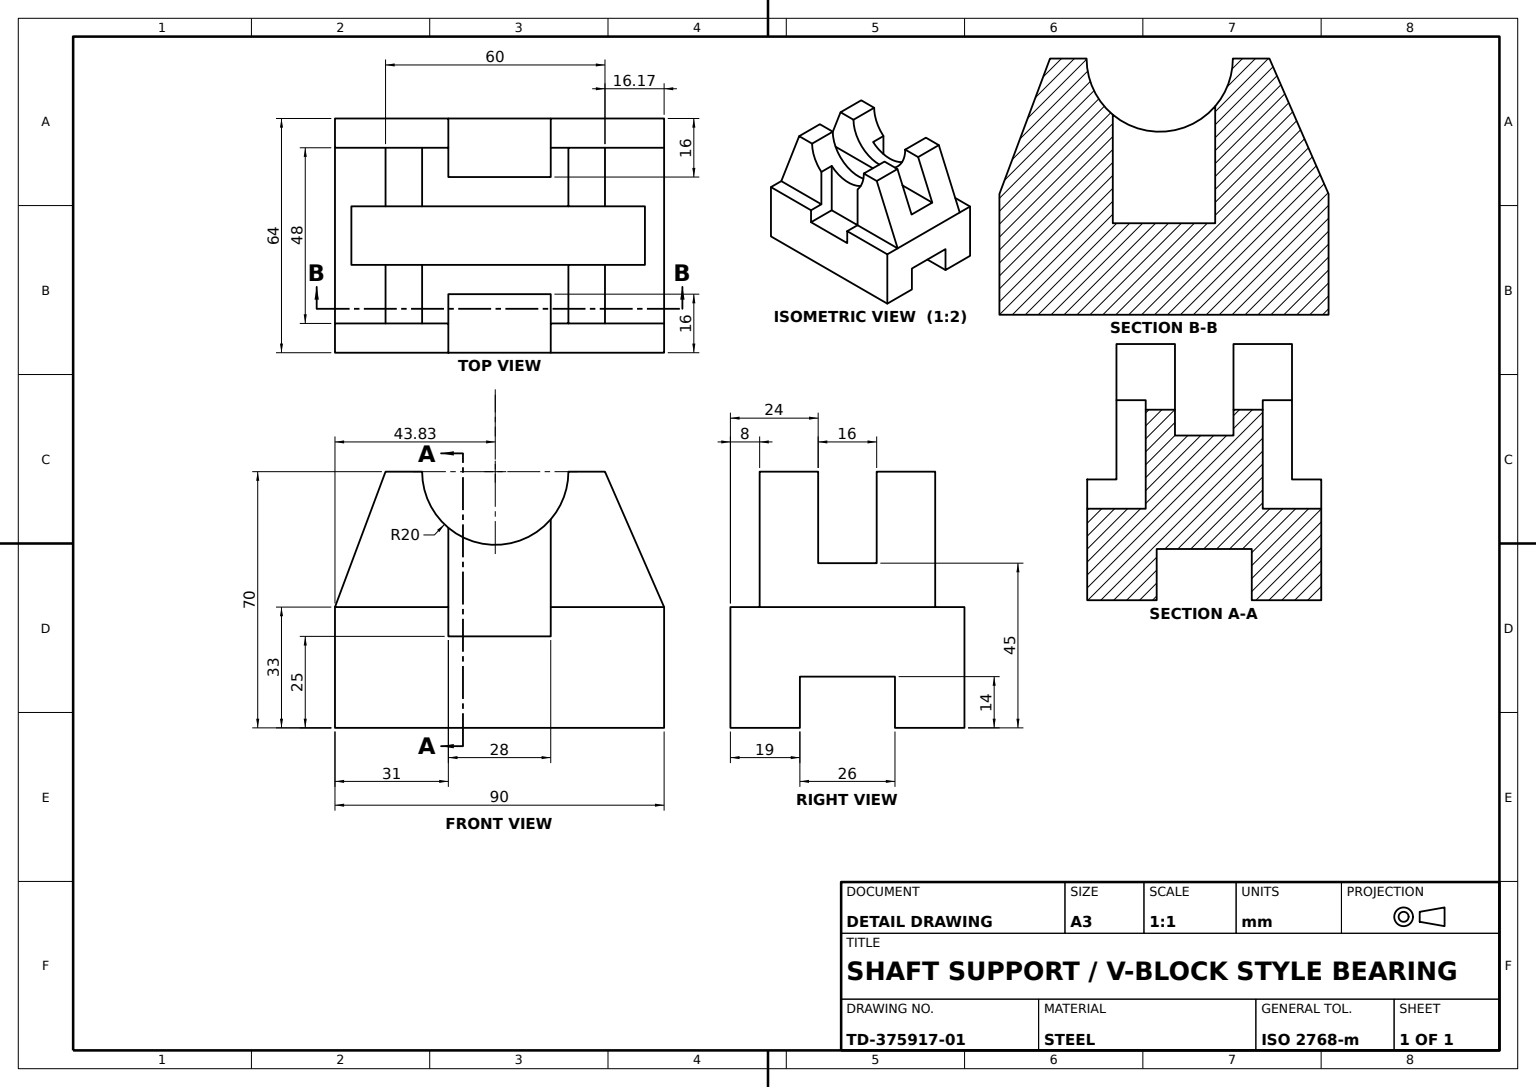
SolidWorks part; units mm, degrees
material "Plain Carbon Steel"
ref_plane "Front Plane" through (0, 0, 0) normal (0, 0, 1) x (1, 0, 0)
ref_plane "Top Plane" through (0, 0, 0) normal (0, 1, 0) x (1, 0, 0)
ref_plane "Right Plane" through (0, 0, 0) normal (1, 0, 0) x (0, 0, -1)
sketch "Base Block Sketch" plane through (0, 0, 0) normal (0, 0, 1) x (1, 0, 0)
  line L1 (0, 0) -> (90, 0)
  line L2 (0, 0) -> (0, 33)
  line L3 (0, 33) -> (90, 33)
  line L4 (90, 0) -> (90, 33)
  dimension "D1" = 90
  dimension "D2" = 33
extrude "Base Block" add sketch "Base Block Sketch" along normal mid plane 64
sketch "Bottom Slot Sketch" plane through (90, 0, 0) normal (1, 0, 0) x (0, 0, -1)
  line L0 (-32, 0) -> (32, 0) construction
  line L1 (-13, 0) -> (13, 0)
  line L2 (-13, 0) -> (-13, 14)
  line L3 (-13, 14) -> (13, 14)
  line L4 (13, 0) -> (13, 14)
  line L5 (0, 0) -> (0, 27.2382) construction
  dimension "D1" = 26
  dimension "D2" = 13
  dimension "D3" = 14
extrude "Bottom Slot" cut sketch "Bottom Slot Sketch" against normal through all
sketch "Support Uprights Sketch" plane through (90, 0, 0) normal (1, 0, 0) x (0, 0, -1)
  line L0 (0, 0) -> (0, 75.595) construction
  line L1 (-32, 33) -> (32, 33) construction
  line L2 (-24, 33) -> (24, 33)
  line L3 (-24, 33) -> (-24, 70)
  line L4 (-24, 70) -> (-8, 70)
  line L5 (24, 33) -> (24, 70)
  line L6 (8, 70) -> (24, 70)
  line L8 (-8, 70) -> (-8, 45)
  line L9 (-8, 45) -> (8, 45)
  line L10 (8, 70) -> (8, 45)
  dimension "D1" = 48
  dimension "D2" = 37
  dimension "D3" = 24
  dimension "D4" = 16
  dimension "D5" = 8
  dimension "D6" = 25
extrude "Support Uprights" add sketch "Support Uprights Sketch" against normal blind 90
sketch "Centre Recess Sketch" plane through (0, 0, 24) normal (0, 0, 1) x (1, 0, 0)
  line L0 (13.8296, 70) -> (73.8296, 70)
  line L1 (0, 70) -> (90, 70) construction
  line L2 (43.8296, 70) -> (43.8296, -5.7343) construction
  line L3 (73.8296, 70) -> (90, 33)
  line L5 (90, 70) -> (90, 33) construction
  line L9 (0, 33) -> (13.8296, 70)
  line L10 (73.8296, 70) -> (90, 70)
  line L11 (90, 70) -> (90, 33)
  line L12 (13.8296, 70) -> (0, 70)
  line L13 (0, 70) -> (0, 33)
  line M6 (90, 33) -> (90, 70)
  line M7 (90, 70) -> (0, 70)
  line M8 (0, 70) -> (0, 33)
  dimension "D1" = 60
  dimension "D2" = 16.1704
extrude "Centre Recess" cut sketch "Centre Recess Sketch" against normal through all contours L3 M7 M6 | L9 M8 M7
sketch "Cradle Arc Sketch" plane through (0, 0, -24) normal (0, 0, -1) x (-1, 0, 0)
  line L0 (-13.8296, 70) -> (-73.8296, 70) construction
  line L1 (-23.8296, 70) -> (-63.8296, 70)
  arc A0 (-63.8296, 70) -> (-23.8296, 70) centre (-43.8296, 70) ccw
  dimension "D1" = 40
extrude "Cradle Arc Cut" cut sketch "Cradle Arc Sketch" against normal through all
sketch "Upright U-Slot Sketch" plane through (0, 70, 0) normal (0, 1, 0) x (1, 0, 0)
  line L0 (45, -32) -> (45, 41.1403) construction
  line L1 (90, -32) -> (0, -32) construction
  line L2 (90, 32) -> (0, 32) construction
  line L3 (31, 32) -> (59, 32)
  line L4 (31, 32) -> (31, 16)
  line L5 (31, 16) -> (59, 16)
  line L6 (59, 32) -> (59, 16)
  line L8 (31, -32) -> (59, -32)
  line L9 (31, -32) -> (31, -16)
  line L10 (31, -16) -> (59, -16)
  line L11 (59, -32) -> (59, -16)
  dimension "D1" = 16
  dimension "D2" = 28
  dimension "D3" = 14
  dimension "D4" = 16
extrude "Upright U-Slot" cut sketch "Upright U-Slot Sketch" against normal blind 45
